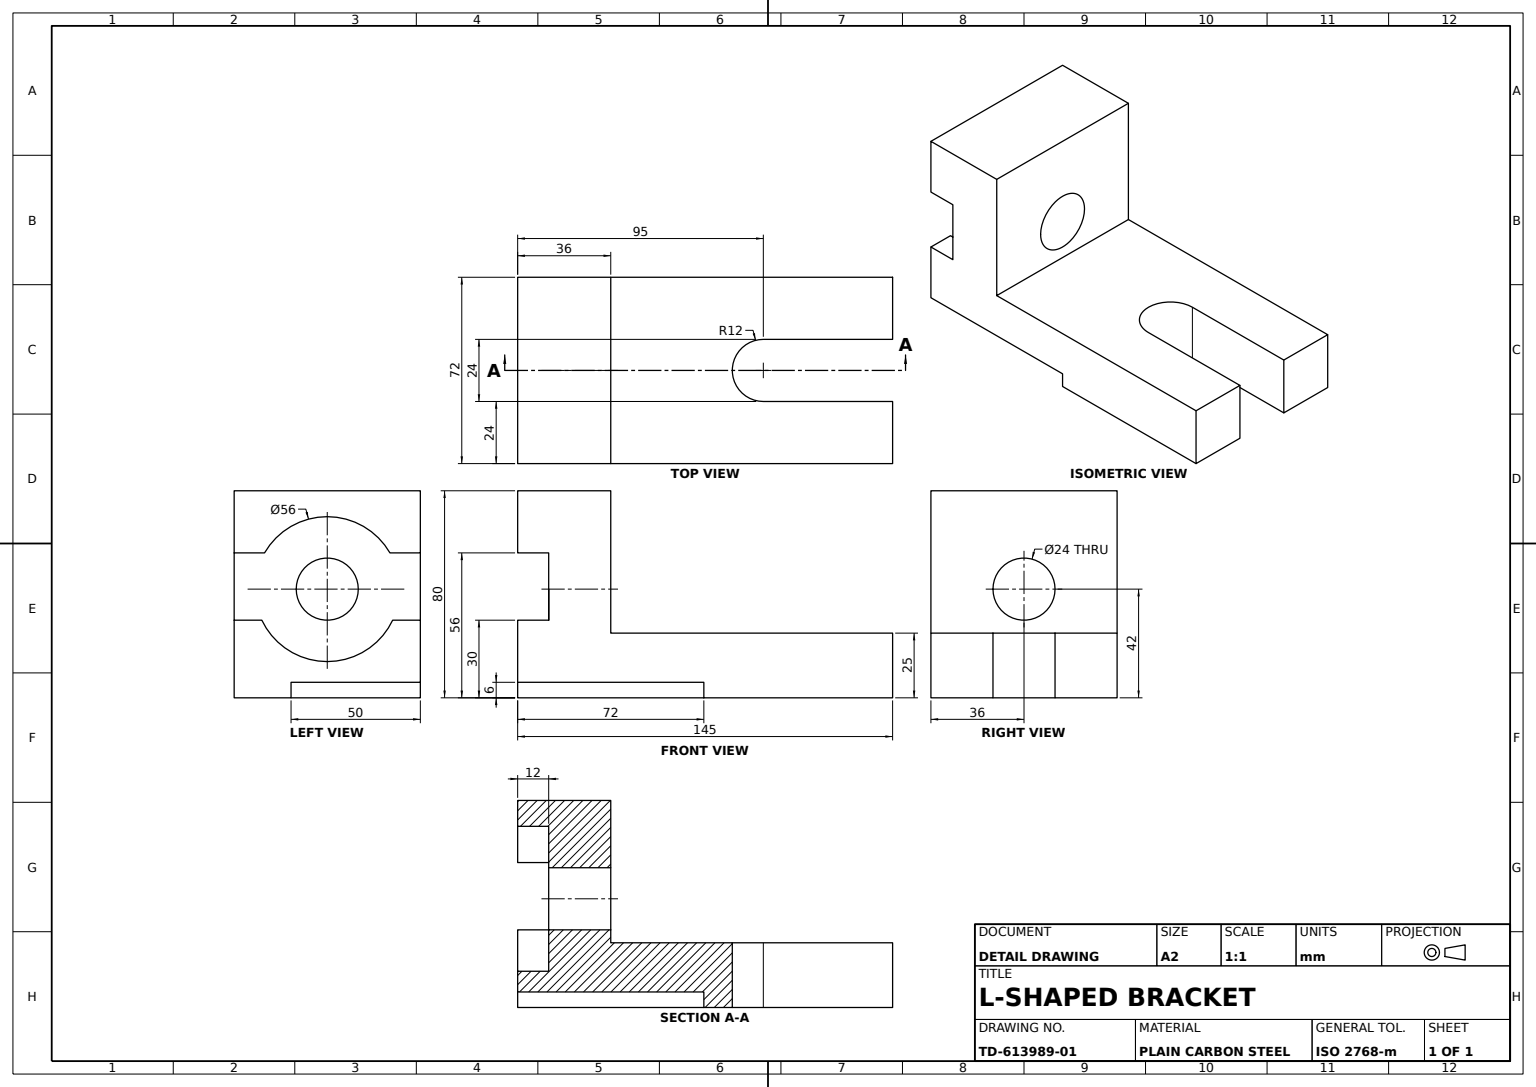
from build123d import *

# Parameters (mm, degrees)
BASE_PLATE_SKETCH_145X72_W  = 145
BASE_PLATE_SKETCH_145X72_H  = 72
BASE_PLATE_25_THICK_DEPTH   = 25
UNDERSIDE_RELIEF_SKETCH_W   = 72
UNDERSIDE_RELIEF_SKETCH_H   = 6
UNDERSIDE_RELIEF_CUT_DEPTH  = 50
CLEVIS_SLOT_CUT_DEPTH       = 50
LOCATING_PAD_SKETCH_W       = 12
LOCATING_PAD_SKETCH_H       = 72
LOCATING_PAD_5_HIGH_DEPTH   = 5
UPRIGHT_BLOCK_72_WIDE_DEPTH = 72
COUNTERBORE_SKETCH_36_R     = 28
COUNTERBORE_36X12_DEPTH     = 12
CROSS_HOLE_SKETCH_24_R      = 12
CROSS_HOLE_24_DEPTH         = 160.32670837


with BuildPart() as part:
    # Base Plate Sketch 145x72 → Base Plate 25 Thick (new body)
    with BuildSketch(Plane(origin=(0, 0, 0), x_dir=(1, 0, 0), z_dir=(0, 1, 0))):
        Rectangle(BASE_PLATE_SKETCH_145X72_W, BASE_PLATE_SKETCH_145X72_H)
    extrude(amount=BASE_PLATE_25_THICK_DEPTH)

    # Underside Relief Sketch → Underside Relief Cut (cut)
    with BuildSketch(Plane.XY.offset(36)):
        with Locations((-36.5, 3)):
            Rectangle(UNDERSIDE_RELIEF_SKETCH_W, UNDERSIDE_RELIEF_SKETCH_H)
    extrude(amount=-UNDERSIDE_RELIEF_CUT_DEPTH, mode=Mode.SUBTRACT)

    # Clevis Slot Sketch 24 Wide → Clevis Slot Cut (cut)
    with BuildSketch(Plane(origin=(0, 25, 0), x_dir=(1, 0, 0), z_dir=(0, 1, 0))):
        with BuildLine():
            Line((22.5, 12), (72.5, 12))
            Line((72.5, 12), (72.5, -12))
            Line((72.5, -12), (22.5, -12))
            ThreePointArc((22.5, -12), (10.5, 0), (22.5, 12))
        make_face()
    extrude(amount=-CLEVIS_SLOT_CUT_DEPTH, mode=Mode.SUBTRACT)

    # Locating Pad Sketch → Locating Pad 5 High (add)
    with BuildSketch(Plane(origin=(0, 25, 0), x_dir=(1, 0, 0), z_dir=(0, 1, 0))):
        with Locations((-66.5, 0)):
            Rectangle(LOCATING_PAD_SKETCH_W, LOCATING_PAD_SKETCH_H)
    extrude(amount=LOCATING_PAD_5_HIGH_DEPTH)

    # Upright Block Profile Sketch → Upright Block 72 Wide (add)
    with BuildSketch(Plane.XY.offset(36)):
        Polygon((-60.5, 25), (-60.5, 56), (-72.5, 56), (-72.5, 80), (-36.5, 80), (-36.5, 25), align=None)
    extrude(amount=-UPRIGHT_BLOCK_72_WIDE_DEPTH)

    # Counterbore Sketch Ø36 → Counterbore Ø36x12 (cut)
    with BuildSketch(Plane.ZY.offset(72.5)):
        with Locations((0, 42)):
            Circle(COUNTERBORE_SKETCH_36_R)
    extrude(amount=-COUNTERBORE_36X12_DEPTH, mode=Mode.SUBTRACT)

    # Cross Hole Sketch Ø24 → Cross Hole Ø24 (cut, through all)
    with BuildSketch(Plane.ZY.offset(60.5)):
        with Locations((0, 42)):
            Circle(CROSS_HOLE_SKETCH_24_R)
    extrude(amount=-CROSS_HOLE_24_DEPTH, mode=Mode.SUBTRACT)


solid = part.part
